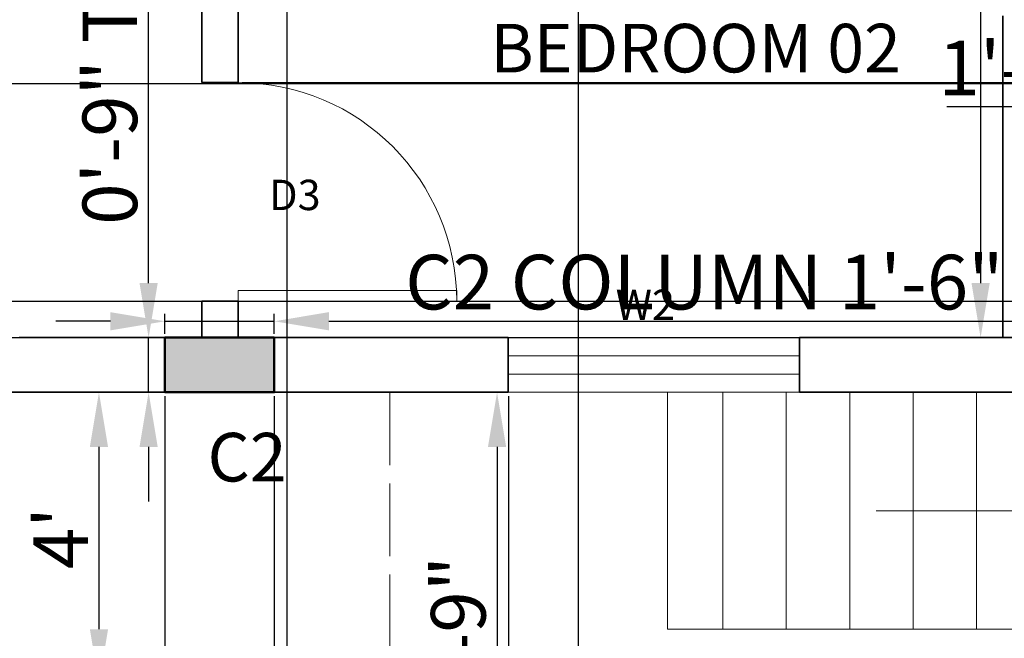
# Model space of a CAD drawing. Units: inches. Extents: x 2621 to 6190, y 513 to 1320.
# Tile 7 of 11: x 2997 to 3160, y 661 to 763. Entities that reach past the tile are written whole.
import ezdxf

# ---------------------------------------------------------------- set-up
doc = ezdxf.new("R2010")
doc.units = ezdxf.units.IN
doc.linetypes.add('ACAD_ISO02W100', pattern=[15, 12, -3])
for name, color, linetype, lineweight in [('A-ANNO-DIMS', 5, 'Continuous', 18), ('A-ANNO-TEXT', 7, 'Continuous', 18), ('A-AREA-IDEN', 7, 'Continuous', 25), ('A-FLOR-PROJ', 1, 'ACAD_ISO02W100', 18), ('A-WALL', 7, 'Continuous', 35), ('columns', 2, 'Continuous', 50), ('door', 1, 'Continuous', 18), ('S-COLS-IDEN', 2, 'Continuous', 25), ('S-COLS-PATT', 2, 'Continuous', 13), ('stairs', 104, 'Continuous', 18), ('window', 172, 'Continuous', 18)]:
    doc.layers.add(name, color=color, linetype=linetype, lineweight=lineweight)
doc.styles.get("Standard").update_dxf_attribs({"font": 'arial.ttf'})
doc.dimstyles.new('ISO-25', dxfattribs={"dimtxt": 9, "dimasz": 9, "dimexe": 1.25, "dimexo": 0.625, "dimtad": 1, "dimlunit": 3, "dimtxsty": 'Standard', "dimcen": 2.5, "dimadec": 0, "dimazin": 0, "dimtfac": 1, "dimtmove": 0, "dimatfit": 3, "dimfxl": 1, "dimarcsym": 0})

# ---------------------------------------------------------------- blocks, each defined once
blk = doc.blocks.new('*U2')
for p, q in [((0, 0), (0, 6)), ((36, 0), (36, 6))]:
    blk.add_line(p, q)
blk.add_lwpolyline([(0, 0), (0, -36), (1.75, -36), (1.75, 0)], close=True)
blk.add_arc((0, 0), 36, 270, 0)
blk = doc.blocks.new('*D28')
at = {"layer": 'A-ANNO-DIMS', "color": 0, "lineweight": -2, "transparency": 16777216}
for p, q in [((3158.76, 890.89), (3154.45, 890.89)), ((3155.7, 881.89), (3155.7, 719.89)), ((3158.76, 710.89), (3154.45, 710.89))]:
    blk.add_line(p, q, dxfattribs=at)
at = {"layer": 'A-ANNO-DIMS', "color": 0, "transparency": 16777216}
for points in [[(3154.2, 881.89), (3157.2, 881.89), (3155.7, 890.89)], [(3154.2, 719.89), (3157.2, 719.89), (3155.7, 710.89)]]:
    blk.add_solid(points, dxfattribs=at)
at = {"layer": 'Defpoints', "color": 0, "transparency": 16777216}
for p in [(3159.38, 890.89), (3155.7, 710.89), (3159.38, 710.89)]:
    blk.add_point(p, dxfattribs=at)
at = {"layer": 'A-ANNO-DIMS', "color": 0, "transparency": 16777216, "insert": (3150.48, 800.89), "char_height": 9, "attachment_point": 5, "rotation": 90}
blk.add_mtext("15'", dxfattribs=at)
blk = doc.blocks.new('*D33')
at = {"layer": 'A-ANNO-DIMS', "color": 0, "lineweight": -2, "transparency": 16777216}
for p, q in [((2997.94, 701.89), (3011.69, 701.89)), ((3010.44, 692.89), (3010.44, 662.89)), ((2997.94, 653.89), (3011.69, 653.89))]:
    blk.add_line(p, q, dxfattribs=at)
at = {"layer": 'A-ANNO-DIMS', "color": 0, "transparency": 16777216}
for points in [[(3008.94, 692.89), (3011.94, 692.89), (3010.44, 701.89)], [(3008.94, 662.89), (3011.94, 662.89), (3010.44, 653.89)]]:
    blk.add_solid(points, dxfattribs=at)
at = {"layer": 'Defpoints', "color": 0, "transparency": 16777216}
for p in [(2997.32, 701.89), (2997.32, 653.89), (3010.44, 653.89)]:
    blk.add_point(p, dxfattribs=at)
at = {"layer": 'A-ANNO-DIMS', "color": 0, "transparency": 16777216, "insert": (3005.32, 677.89), "char_height": 9, "attachment_point": 5, "rotation": 90}
blk.add_mtext("4'", dxfattribs=at)
blk = doc.blocks.new('*D34')
at = {"layer": 'A-ANNO-DIMS', "color": 0, "lineweight": -2, "transparency": 16777216}
for p, q in [((3058.97, 701.89), (3077.28, 701.89)), ((3076.03, 692.89), (3076.03, 629.89)), ((3058.97, 620.89), (3077.28, 620.89))]:
    blk.add_line(p, q, dxfattribs=at)
at = {"layer": 'A-ANNO-DIMS', "color": 0, "transparency": 16777216}
for points in [[(3074.53, 692.89), (3077.53, 692.89), (3076.03, 701.89)], [(3074.53, 629.89), (3077.53, 629.89), (3076.03, 620.89)]]:
    blk.add_solid(points, dxfattribs=at)
at = {"layer": 'Defpoints', "color": 0, "transparency": 16777216}
for p in [(3058.34, 701.89), (3058.34, 620.89), (3076.03, 620.89)]:
    blk.add_point(p, dxfattribs=at)
at = {"layer": 'A-ANNO-DIMS', "color": 0, "transparency": 16777216, "insert": (3070.81, 661.39), "char_height": 9, "attachment_point": 5, "rotation": 90}
blk.add_mtext('6\'-9"', dxfattribs=at)
blk = doc.blocks.new('WIN-48IN')
for p, q in [((48, 9), (0, 9)), ((0, 9), (0, 0)), ((48, 0), (48, 9)), ((0, 6), (48, 6)), ((0, 3), (48, 3)), ((0, 0), (48, 0))]:
    blk.add_line(p, q)
blk = doc.blocks.new('COL-C2-9X18')
blk.add_lwpolyline([(18, 9), (18, 0), (0, 0), (0, 9)], close=True)
blk = doc.blocks.new('*D53')
at = {"layer": 'A-ANNO-DIMS', "color": 0, "lineweight": -2, "transparency": 16777216}
for p, q in [((3021.32, 711.51), (3021.32, 714.84)), ((3039.32, 711.51), (3039.32, 714.84)), ((3012.32, 713.59), (3003.32, 713.59)), ((3021.32, 713.59), (3039.32, 713.59)), ((3048.32, 713.59), (3190.87, 713.59))]:
    blk.add_line(p, q, dxfattribs=at)
at = {"layer": 'A-ANNO-DIMS', "color": 0, "transparency": 16777216}
for points in [[(3012.32, 715.09), (3012.32, 712.09), (3021.32, 713.59)], [(3048.32, 715.09), (3048.32, 712.09), (3039.32, 713.59)]]:
    blk.add_solid(points, dxfattribs=at)
at = {"layer": 'Defpoints', "color": 0, "transparency": 16777216}
for p in [(3039.32, 713.59), (3021.32, 710.89), (3039.32, 710.89)]:
    blk.add_point(p, dxfattribs=at)
at = {"layer": 'A-ANNO-DIMS', "color": 0, "transparency": 16777216, "insert": (3124.09, 718.87), "char_height": 9, "attachment_point": 5}
blk.add_mtext('C2 COLUMN 1\'-6" TYP.', dxfattribs=at)
blk = doc.blocks.new('*D54')
at = {"layer": 'A-ANNO-DIMS', "color": 0, "lineweight": -2, "transparency": 16777216}
for p, q in [((3018.62, 719.89), (3018.62, 785)), ((3020.69, 710.89), (3017.37, 710.89)), ((3018.62, 701.89), (3018.62, 710.89)), ((3020.69, 701.89), (3017.37, 701.89)), ((3018.62, 692.89), (3018.62, 683.89))]:
    blk.add_line(p, q, dxfattribs=at)
at = {"layer": 'A-ANNO-DIMS', "color": 0, "transparency": 16777216}
for points in [[(3017.12, 719.89), (3020.12, 719.89), (3018.62, 710.89)], [(3017.12, 692.89), (3020.12, 692.89), (3018.62, 701.89)]]:
    blk.add_solid(points, dxfattribs=at)
at = {"layer": 'Defpoints', "color": 0, "transparency": 16777216}
for p in [(3018.62, 710.89), (3021.32, 710.89), (3021.32, 701.89)]:
    blk.add_point(p, dxfattribs=at)
at = {"layer": 'A-ANNO-DIMS', "color": 0, "transparency": 16777216, "insert": (3013.4, 756.94), "char_height": 9, "attachment_point": 5, "rotation": 90}
blk.add_mtext('0\'-9" TYP.', dxfattribs=at)
blk = doc.blocks.new('*D72')
at = {"layer": 'A-ANNO-DIMS', "color": 0, "lineweight": -2, "transparency": 16777216}
for p, q in [((3183.49, 744.56), (3183.49, 750.14)), ((3204.49, 744.56), (3204.49, 750.14)), ((3183.49, 748.89), (3150.16, 748.89)), ((3195.49, 748.89), (3192.49, 748.89))]:
    blk.add_line(p, q, dxfattribs=at)
at = {"layer": 'A-ANNO-DIMS', "color": 0, "transparency": 16777216}
for points in [[(3192.49, 750.39), (3192.49, 747.39), (3183.49, 748.89)], [(3195.49, 750.39), (3195.49, 747.39), (3204.49, 748.89)]]:
    blk.add_solid(points, dxfattribs=at)
at = {"layer": 'Defpoints', "color": 0, "transparency": 16777216}
for p in [(3183.49, 748.89), (3183.49, 743.94), (3204.49, 743.94)]:
    blk.add_point(p, dxfattribs=at)
at = {"layer": 'A-ANNO-DIMS', "color": 0, "transparency": 16777216, "insert": (3162.32, 754.11), "char_height": 9, "attachment_point": 5}
blk.add_mtext('1\'-9"', dxfattribs=at)
blk = doc.blocks.new('*D82')
at = {"layer": 'A-ANNO-DIMS', "color": 0, "lineweight": -2, "transparency": 16777216}
for p, q in [((2924.85, 889.24), (3291.63, 889.24)), ((3290.38, 719.89), (3290.38, 880.24)), ((2917.49, 710.89), (3291.63, 710.89))]:
    blk.add_line(p, q, dxfattribs=at)
at = {"layer": 'A-ANNO-DIMS', "color": 0, "transparency": 16777216}
for points in [[(3288.88, 880.24), (3291.88, 880.24), (3290.38, 889.24)], [(3288.88, 719.89), (3291.88, 719.89), (3290.38, 710.89)]]:
    blk.add_solid(points, dxfattribs=at)
at = {"layer": 'Defpoints', "color": 0, "transparency": 16777216}
for p in [(2924.22, 889.24), (3290.38, 889.24), (2916.87, 710.89)]:
    blk.add_point(p, dxfattribs=at)
at = {"layer": 'A-ANNO-DIMS', "color": 0, "transparency": 16777216, "insert": (3285.1, 800.07), "char_height": 9, "attachment_point": 5, "rotation": 90}
blk.add_mtext('14\'-10 1/2"', dxfattribs=at)
blk = doc.blocks.new('*D86')
at = {"layer": 'A-ANNO-DIMS', "color": 0, "lineweight": -2, "transparency": 16777216}
for p, q in [((2898.87, 701.26), (2898.87, 519.64)), ((3021.32, 701.26), (3021.32, 519.64)), ((2907.87, 520.89), (3012.32, 520.89))]:
    blk.add_line(p, q, dxfattribs=at)
at = {"layer": 'A-ANNO-DIMS', "color": 0, "transparency": 16777216}
for points in [[(2907.87, 522.39), (2907.87, 519.39), (2898.87, 520.89)], [(3012.32, 522.39), (3012.32, 519.39), (3021.32, 520.89)]]:
    blk.add_solid(points, dxfattribs=at)
at = {"layer": 'Defpoints', "color": 0, "transparency": 16777216}
for p in [(2898.87, 701.89), (3021.32, 701.89), (3021.32, 520.89)]:
    blk.add_point(p, dxfattribs=at)
at = {"layer": 'A-ANNO-DIMS', "color": 0, "transparency": 16777216, "insert": (2960.09, 526.17), "char_height": 9, "attachment_point": 5}
blk.add_mtext('10\'-2 1/2"', dxfattribs=at)
blk = doc.blocks.new('*D92')
at = {"layer": 'A-ANNO-DIMS', "color": 0, "lineweight": -2, "transparency": 16777216}
for p, q in [((3222.38, 701.26), (3222.38, 519.64)), ((2730.38, 686.26), (2730.38, 519.64)), ((2739.38, 520.89), (3213.38, 520.89))]:
    blk.add_line(p, q, dxfattribs=at)
at = {"layer": 'A-ANNO-DIMS', "color": 0, "transparency": 16777216}
for points in [[(2739.38, 522.39), (2739.38, 519.39), (2730.38, 520.89)], [(3213.38, 522.39), (3213.38, 519.39), (3222.38, 520.89)]]:
    blk.add_solid(points, dxfattribs=at)
at = {"layer": 'Defpoints', "color": 0, "transparency": 16777216}
for p in [(3222.38, 701.89), (2730.38, 686.89), (3222.38, 520.89)]:
    blk.add_point(p, dxfattribs=at)
at = {"layer": 'A-ANNO-DIMS', "color": 0, "transparency": 16777216, "insert": (2976.38, 526.11), "char_height": 9, "attachment_point": 5}
blk.add_mtext('41\'-0"', dxfattribs=at)
blk = doc.blocks.new('*D95')
at = {"layer": 'A-ANNO-DIMS', "color": 0, "lineweight": -2, "transparency": 16777216}
for p, q in [((2788.01, 752.76), (3291.63, 752.76)), ((3290.38, 725.89), (3290.38, 743.76)), ((2788.01, 716.89), (3291.63, 716.89))]:
    blk.add_line(p, q, dxfattribs=at)
at = {"layer": 'A-ANNO-DIMS', "color": 0, "transparency": 16777216}
for points in [[(3288.88, 743.76), (3291.88, 743.76), (3290.38, 752.76)], [(3288.88, 725.89), (3291.88, 725.89), (3290.38, 716.89)]]:
    blk.add_solid(points, dxfattribs=at)
at = {"layer": 'Defpoints', "color": 0, "transparency": 16777216}
for p in [(2787.38, 752.76), (3290.38, 752.76), (2787.38, 716.89)]:
    blk.add_point(p, dxfattribs=at)
at = {"layer": 'A-ANNO-DIMS', "color": 0, "transparency": 16777216, "insert": (3285.16, 734.83), "char_height": 9, "attachment_point": 5, "rotation": 90}
blk.add_mtext('3\'-0"', dxfattribs=at)
blk = doc.blocks.new('*D96')
at = {"layer": 'A-ANNO-DIMS', "color": 0, "lineweight": -2, "transparency": 16777216}
for p, q in [((3034.01, 752.89), (3291.63, 752.89)), ((3290.38, 725.89), (3290.38, 743.89)), ((3034.01, 716.89), (3291.63, 716.89))]:
    blk.add_line(p, q, dxfattribs=at)
at = {"layer": 'A-ANNO-DIMS', "color": 0, "transparency": 16777216}
for points in [[(3288.88, 743.89), (3291.88, 743.89), (3290.38, 752.89)], [(3288.88, 725.89), (3291.88, 725.89), (3290.38, 716.89)]]:
    blk.add_solid(points, dxfattribs=at)
at = {"layer": 'Defpoints', "color": 0, "transparency": 16777216}
for p in [(3033.38, 752.89), (3290.38, 752.89), (3033.38, 716.89)]:
    blk.add_point(p, dxfattribs=at)
at = {"layer": 'A-ANNO-DIMS', "color": 0, "transparency": 16777216, "insert": (3285.16, 734.89), "char_height": 9, "attachment_point": 5, "rotation": 90}
blk.add_mtext('3\'-0"', dxfattribs=at)
blk = doc.blocks.new('*D102')
at = {"layer": 'A-ANNO-DIMS', "color": 0, "lineweight": -2, "transparency": 16777216}
for p, q in [((2915.57, 1054.4), (2915.57, 519.64)), ((2942.88, 1054.4), (2942.88, 519.64)), ((2924.57, 520.89), (2933.88, 520.89)), ((2942.88, 520.89), (2998.18, 520.89))]:
    blk.add_line(p, q, dxfattribs=at)
at = {"layer": 'A-ANNO-DIMS', "color": 0, "transparency": 16777216}
for points in [[(2924.57, 522.39), (2924.57, 519.39), (2915.57, 520.89)], [(2933.88, 522.39), (2933.88, 519.39), (2942.88, 520.89)]]:
    blk.add_solid(points, dxfattribs=at)
at = {"layer": 'Defpoints', "color": 0, "transparency": 16777216}
for p in [(2915.57, 1055.03), (2942.88, 1055.03), (2942.88, 520.89)]:
    blk.add_point(p, dxfattribs=at)
at = {"layer": 'A-ANNO-DIMS', "color": 0, "transparency": 16777216, "insert": (2975.03, 526.17), "char_height": 9, "attachment_point": 5}
blk.add_mtext('2\'-3 1/2"', dxfattribs=at)
blk = doc.blocks.new('*D107')
at = {"layer": 'A-ANNO-DIMS', "color": 0, "lineweight": -2, "transparency": 16777216}
for p, q in [((3041.38, 1076.26), (3041.38, 519.64)), ((3089.38, 1076.26), (3089.38, 519.64)), ((3050.38, 520.89), (3080.38, 520.89))]:
    blk.add_line(p, q, dxfattribs=at)
at = {"layer": 'A-ANNO-DIMS', "color": 0, "transparency": 16777216}
for points in [[(3050.38, 522.39), (3050.38, 519.39), (3041.38, 520.89)], [(3080.38, 522.39), (3080.38, 519.39), (3089.38, 520.89)]]:
    blk.add_solid(points, dxfattribs=at)
at = {"layer": 'Defpoints', "color": 0, "transparency": 16777216}
for p in [(3041.38, 1076.89), (3089.38, 1076.89), (3089.38, 520.89)]:
    blk.add_point(p, dxfattribs=at)
at = {"layer": 'A-ANNO-DIMS', "color": 0, "transparency": 16777216, "insert": (3065.38, 526.11), "char_height": 9, "attachment_point": 5}
blk.add_mtext('4\'-0"', dxfattribs=at)
blk = doc.blocks.new('*D108')
at = {"layer": 'A-ANNO-DIMS', "color": 0, "lineweight": -2, "transparency": 16777216}
for p, q in [((3039.32, 701.26), (3039.32, 519.64)), ((3077.89, 701.26), (3077.89, 519.64)), ((3048.32, 520.89), (3068.89, 520.89)), ((3077.89, 520.89), (3133.03, 520.89))]:
    blk.add_line(p, q, dxfattribs=at)
at = {"layer": 'A-ANNO-DIMS', "color": 0, "transparency": 16777216}
for points in [[(3048.32, 522.39), (3048.32, 519.39), (3039.32, 520.89)], [(3068.89, 522.39), (3068.89, 519.39), (3077.89, 520.89)]]:
    blk.add_solid(points, dxfattribs=at)
at = {"layer": 'Defpoints', "color": 0, "transparency": 16777216}
for p in [(3039.32, 701.89), (3077.89, 701.89), (3077.89, 520.89)]:
    blk.add_point(p, dxfattribs=at)
at = {"layer": 'A-ANNO-DIMS', "color": 0, "transparency": 16777216, "insert": (3109.96, 526.17), "char_height": 9, "attachment_point": 5}
blk.add_mtext('3\'-2 1/2"', dxfattribs=at)

msp = doc.modelspace()

# ---------------------------------------------------------------- hatches: boundary and pattern name
at = {"layer": 'S-COLS-PATT'}
h = msp.add_hatch(color=256, dxfattribs=at)
h.dxf.hatch_style = 1
h.paths.add_polyline_path([(2787.381, 1085.89), (2778.381, 1085.89), (2778.381, 1071.89), (2787.381, 1071.89)])
h.paths.add_polyline_path([(3222.381, 1085.89), (3208.381, 1085.89), (3208.381, 1076.89), (3222.381, 1076.89)])
h.paths.add_polyline_path([(3041.381, 1085.89), (3027.381, 1085.89), (3027.381, 1076.89), (3041.381, 1076.89)])
h.paths.add_polyline_path([(2916.381, 1085.89), (2907.381, 1085.89), (2907.381, 1076.89), (2916.381, 1076.89)])
h.paths.add_polyline_path([(2916.381, 1076.89), (2913.381, 1076.89), (2913.381, 1071.89), (2916.381, 1071.89)])
h.paths.add_polyline_path([(2913.381, 1076.89), (2907.381, 1076.89), (2907.381, 1071.89), (2913.381, 1071.89)])
h.paths.add_polyline_path([(2787.381, 896.89), (2778.381, 896.89), (2778.381, 882.89), (2787.381, 882.89)])
h.paths.add_polyline_path([(2924.221, 898.241), (2910.221, 898.241), (2910.221, 889.241), (2924.221, 889.241)])
h.paths.add_polyline_path([(3036.381, 896.89), (3033.381, 896.89), (3027.381, 897.385), (3027.381, 883.385), (3033.381, 883.385), (3033.381, 890.89), (3036.381, 890.89)])
h.paths.add_polyline_path([(3036.381, 890.89), (3033.381, 890.89), (3033.381, 883.385), (3036.381, 883.385)], flags=17)
h.paths.add_polyline_path([(3222.381, 897.745), (3213.381, 897.745), (3213.381, 883.745), (3222.381, 883.745)])
h.paths.add_polyline_path([(3222.381, 710.89), (3208.381, 710.89), (3208.381, 701.89), (3222.381, 701.89)])
h.paths.add_polyline_path([(3039.318, 710.89), (3021.318, 710.89), (3021.318, 701.89), (3039.318, 701.89)])
h.paths.add_polyline_path([(2796.381, 710.89), (2778.381, 710.89), (2778.381, 701.89), (2796.381, 701.89)])

# ---------------------------------------------------------------- linework, layer by layer
at = {"layer": 'A-FLOR-PROJ'}
msp.add_lwpolyline([(3058.344, 701.89), (3058.344, 620.89), (2730.381, 620.89), (2730.381, 782.89)], dxfattribs=at)
at = {"layer": 'A-WALL'}
for p, q in [((3027.381, 902.548), (3027.381, 752.89)), ((3033.381, 883.385), (3033.381, 752.89)), ((3159.381, 710.89), (3159.381, 763.89)), ((3033.381, 752.89), (3027.381, 752.89)), ((3033.381, 716.89), (3027.381, 716.89)), ((3027.381, 716.89), (3027.381, 710.89)), ((3033.381, 716.89), (3033.381, 710.89)), ((2997.318, 710.89), (3077.887, 710.89)), ((3077.887, 710.89), (3077.887, 701.89)), ((3125.887, 710.89), (3125.887, 701.89)), ((3125.887, 710.89), (3213.381, 710.89)), ((2868.381, 701.89), (3077.887, 701.89)), ((3125.887, 701.89), (3222.381, 701.89))]:
    msp.add_line(p, q, dxfattribs=at)
at = {"layer": 'stairs'}
for p, q in [((3104.102, 701.89), (3104.102, 662.89)), ((3113.244, 701.89), (3113.244, 662.89)), ((3123.692, 701.89), (3123.692, 662.89)), ((3134.14, 701.89), (3134.14, 662.89)), ((3144.589, 701.89), (3144.589, 662.89)), ((3155.037, 701.89), (3155.037, 662.89)), ((3204.871, 682.39), (3138.49, 682.39)), ((3186.381, 662.89), (3104.102, 662.89))]:
    msp.add_line(p, q, dxfattribs=at)

# ---------------------------------------------------------------- block references
at = {"layer": 'columns'}
msp.add_blockref('COL-C2-9X18', (3021.318, 701.89), dxfattribs=at)
at = {"layer": 'door', "rotation": 90}
msp.add_blockref('*U2', (3033.381, 716.89), dxfattribs=at)
at = {"layer": 'window'}
msp.add_blockref('WIN-48IN', (3077.887, 701.89), dxfattribs=at)

# ---------------------------------------------------------------- texts
at = {"layer": 'A-ANNO-TEXT', "char_height": 5, "attachment_point": 1}
for s, width, insert in [('D3', 12.30066, (3038.482, 736.893)), ('W2', 21.64382, (3095.572, 718.815))]:
    msp.add_mtext_dynamic_manual_height_columns(s, width=width, gutter_width=12.5, heights=[0], dxfattribs=dict(at, insert=insert))
at = {"layer": 'A-AREA-IDEN', "insert": (3074.901, 762.563), "char_height": 8, "attachment_point": 1}
msp.add_mtext_dynamic_manual_height_columns('BEDROOM 02', width=74.69403, gutter_width=12.5, heights=[0], dxfattribs=at)
at = {"layer": 'S-COLS-IDEN', "insert": (3028.333, 695.21), "char_height": 8, "attachment_point": 1}
msp.add_mtext_dynamic_manual_height_columns('C2', width=53.01391, gutter_width=12.5, heights=[0], dxfattribs=at)

# ---------------------------------------------------------------- dimensions: what is measured, and where the dimension line sits
at = {"layer": 'A-ANNO-DIMS'}
for base, p1, p2, picture, middle in [((3089.381, 520.89), (3041.381, 1076.89), (3089.381, 1076.89), '*D107', (3065.381, 526.11)), ((2942.877, 520.89), (2915.573, 1055.025), (2942.877, 1055.025), '*D102', (2975.027, 526.171)), ((3222.381, 520.89), (2730.381, 686.89), (3222.381, 701.89), '*D92', (2976.381, 526.11)), ((3021.318, 520.89), (2898.869, 701.89), (3021.318, 701.89), '*D86', (2960.094, 526.168)), ((3077.887, 520.89), (3039.318, 701.89), (3077.887, 701.89), '*D108', (3109.957, 526.171))]:
    dim = msp.add_linear_dim(base=base, p1=p1, p2=p2, dimstyle='ISO-25', override={"dimdec": 1, "dimlfac": 1, "dimrnd": 0, "dimzin": 1, "dimdsep": 46, "dimlunit": 4, "dimfrac": 2}, dxfattribs=at)
    dim.commit()
    dim.dimension.update_dxf_attribs({"geometry": picture, "text_midpoint": middle})
for base, p1, p2, angle, override, picture, middle in [((3155.695, 710.89), (3159.381, 890.89), (3159.381, 710.89), 90, {"dimclrd": 0, "dimclre": 0, "dimclrt": 0}, '*D28', (3150.475, 800.89)), ((3290.381, 889.241), (2916.869, 710.89), (2924.221, 889.241), 90, {"dimdec": 1, "dimlfac": 1, "dimrnd": 0, "dimzin": 1, "dimdsep": 46, "dimlunit": 4, "dimfrac": 2}, '*D82', (3285.103, 800.065)), ((3183.488, 748.893), (3204.488, 743.936), (3183.488, 743.936), 180, {"dimdec": 1, "dimlfac": 1, "dimrnd": 0, "dimzin": 1, "dimdsep": 46, "dimlunit": 4, "dimfrac": 2}, '*D72', (3162.324, 754.113)), ((3290.381, 752.764), (2787.381, 716.89), (2787.381, 752.764), 90, {"dimdec": 1, "dimlfac": 1, "dimrnd": 0, "dimzin": 1, "dimdsep": 46, "dimlunit": 4, "dimfrac": 2}, '*D95', (3285.158, 734.827)), ((3290.381, 752.89), (3033.381, 716.89), (3033.381, 752.89), 90, {"dimdec": 1, "dimlfac": 1, "dimrnd": 0, "dimzin": 1, "dimdsep": 46, "dimlunit": 4, "dimfrac": 2}, '*D96', (3285.158, 734.89)), ((3010.445, 653.89), (2997.318, 701.89), (2997.318, 653.89), 90, {"dimclrd": 0, "dimclre": 0, "dimclrt": 0}, '*D33', (3005.32, 677.89)), ((3076.033, 620.89), (3058.344, 701.89), (3058.344, 620.89), 90, {"dimclrd": 0, "dimclre": 0, "dimclrt": 0}, '*D34', (3070.812, 661.39))]:
    dim = msp.add_linear_dim(base=base, p1=p1, p2=p2, angle=angle, dimstyle='ISO-25', override=override, dxfattribs=at)
    dim.commit()
    dim.dimension.update_dxf_attribs({"geometry": picture, "text_midpoint": middle})
dim = msp.add_linear_dim(base=(3018.618, 710.89), p1=(3021.318, 701.89), p2=(3021.318, 710.89), angle=90, text='<> TYP.', dimstyle='ISO-25', override={"dimdec": 1, "dimlfac": 1, "dimrnd": 0, "dimzin": 1, "dimdsep": 46, "dimlunit": 4, "dimfrac": 2}, dxfattribs=at)
dim.commit()
dim.dimension.update_dxf_attribs({"geometry": '*D54', "text_midpoint": (3013.398, 756.944)})
dim = msp.add_linear_dim(base=(3039.318, 713.59), p1=(3021.318, 710.89), p2=(3039.318, 710.89), text='C2 COLUMN <> TYP.', dimstyle='ISO-25', override={"dimdec": 1, "dimlfac": 1, "dimrnd": 0, "dimzin": 1, "dimdsep": 46, "dimlunit": 4, "dimfrac": 2}, dxfattribs=at)
dim.commit()
dim.dimension.update_dxf_attribs({"geometry": '*D53', "text_midpoint": (3124.092, 718.871)})

doc.saveas('drawing.dxf')
